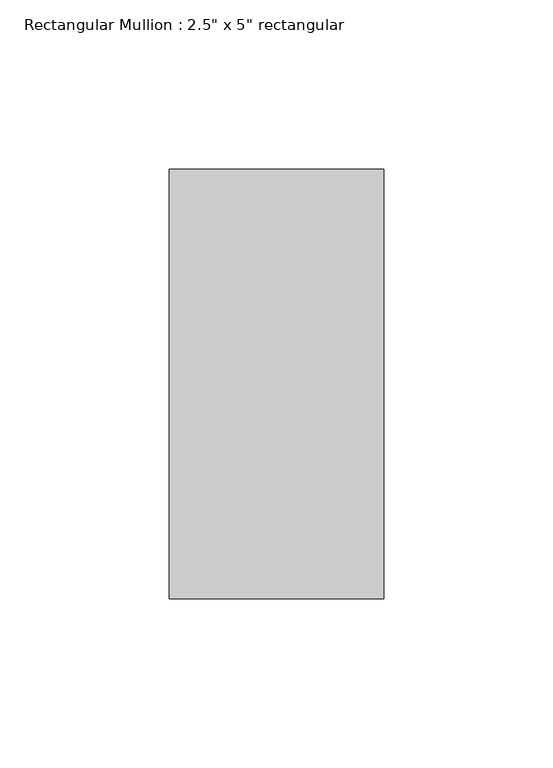
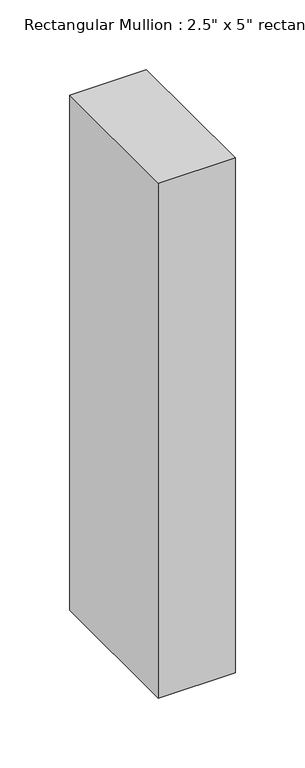
"""IFC4 building model written with IfcOpenShell, lengths in millimetres: member geometry."""

from ifc_helpers import new_model, si_unit, frame, origin, place, context, project, spatial, polyline, outline, extrude, source, transform, mapped, element, save


def member_969ca954(model_context):
    return source(origin(), model_context, "Body", "SweptSolid", [
        extrude(outline(polyline([(0.0, 63.5), (0.0, -63.5), (-63.5, -63.5), (-63.5, 63.5), (0.0, 63.5)])), frame((0.0, 0.0, -450.85), z_axis=(0.0, 0.0, 1.0), x_axis=(1.0, 0.0, 0.0)), (0.0, 0.0, 1.0), 450.85),
    ])


if __name__ == "__main__":
    model = new_model("IFC4")
    model_context = context("Model", 3, world=origin())
    ifc_project = project(units=[si_unit("LENGTHUNIT", "METRE", prefix="MILLI")], contexts=[model_context])
    site = spatial("IfcSite", under=ifc_project)
    building = spatial("IfcBuilding", under=site)
    placement = place(None, origin())
    member_shape = member_969ca954(model_context)
    element("IfcMember", 1, ObjectType="Rectangular Mullion : 2.5\" x 5\" rectangular", at=placement, inside=building, context=model_context, shape_type="MappedRepresentation", body=[
        mapped(member_shape, transform((0.0, 0.0, 0.0), x_axis=(1.0, 0.0, 0.0), y_axis=(0.0, 1.0, 0.0), z_axis=(0.0, 0.0, 1.0))),
    ])
    save(model, "model.ifc")

# Revit data of these elements
# Type "Rectangular Mullion : 2.5\" x 5\" rectangular"
#   built-in parameter 1007304 = 0.416667 (stored number, unit not read)
#   built-in parameter 1007301 = 0.104167 (stored number, unit not read)
#   built-in parameter 1007300 = 0.104167 (stored number, unit not read)
# Element 1 (IfcMember, "Rectangular Mullion : 2.5\" x 5\" rectangular")
#   Materials on its faces: "Aluminum"
# Materials
#   "Aluminum": class "Metal", colour RGB 247 247 247, transparency 0, Description = "Aluminum 6061", Cost = 0
